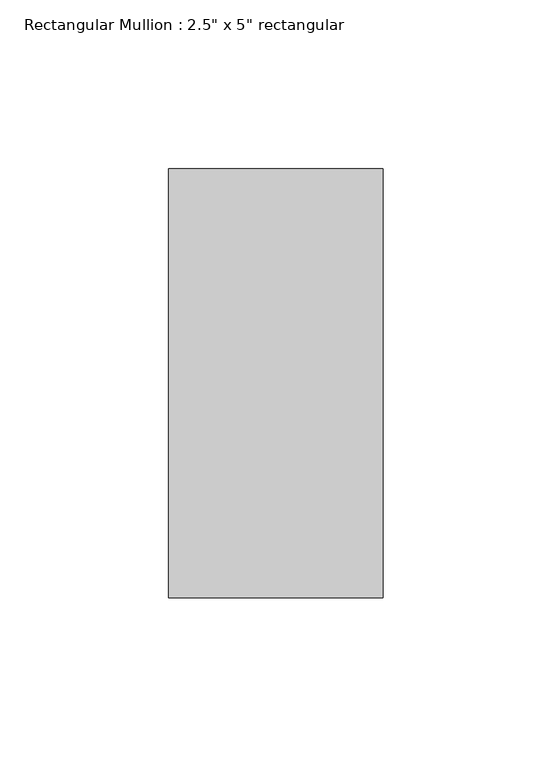
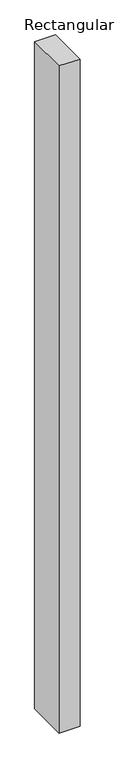
"""IFC4 building model written with IfcOpenShell, lengths in millimetres: member geometry."""

from ifc_helpers import new_model, si_unit, frame, origin, place, context, project, spatial, polyline, outline, extrude, source, transform, mapped, element, save


def member_a7b41546(model_context):
    return source(origin(), model_context, "Body", "SweptSolid", [
        extrude(outline(polyline([(0.0, 63.5), (0.0, -63.5), (-63.5, -63.5), (-63.5, 63.5), (0.0, 63.5)])), frame((0.0, 0.0, -2130.0999183), z_axis=(0.0, 0.0, 1.0), x_axis=(1.0, 0.0, 0.0)), (0.0, 0.0, 1.0), 2130.0999183),
    ])


if __name__ == "__main__":
    model = new_model("IFC4")
    model_context = context("Model", 3, world=origin())
    ifc_project = project(units=[si_unit("LENGTHUNIT", "METRE", prefix="MILLI")], contexts=[model_context])
    site = spatial("IfcSite", under=ifc_project)
    building = spatial("IfcBuilding", under=site)
    placement = place(None, origin())
    member_shape = member_a7b41546(model_context)
    element("IfcMember", 1, ObjectType="Rectangular Mullion : 2.5\" x 5\" rectangular", at=placement, inside=building, context=model_context, shape_type="MappedRepresentation", body=[
        mapped(member_shape, transform((0.0, 0.0, 0.0), x_axis=(1.0, 0.0, 0.0), y_axis=(0.0, 1.0, 0.0), z_axis=(0.0, 0.0, 1.0))),
    ])
    save(model, "model.ifc")

# Revit data of these elements
# Type "Rectangular Mullion : 2.5\" x 5\" rectangular"
#   built-in parameter 1007304 = 0.416667 (stored number, unit not read)
#   built-in parameter 1007301 = 0.104167 (stored number, unit not read)
#   built-in parameter 1007300 = 0.104167 (stored number, unit not read)
# Element 1 (IfcMember, "Rectangular Mullion : 2.5\" x 5\" rectangular")
#   Materials on its faces: "Aluminum"
# Materials
#   "Aluminum": class "Metal", colour RGB 247 247 247, transparency 0, Description = "Aluminum 6061", Cost = 0
